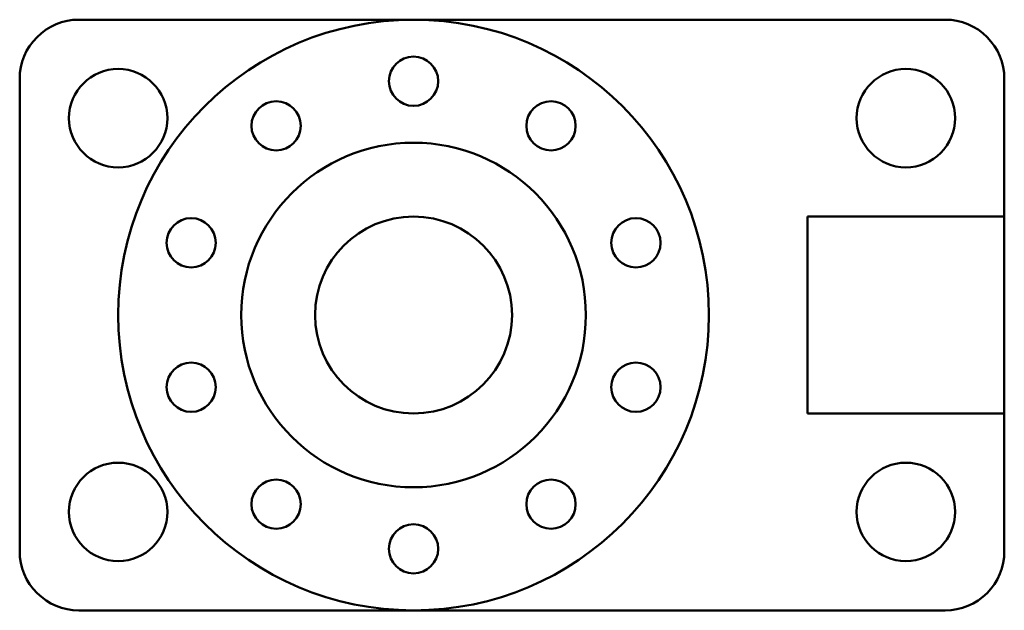
# Model space of a CAD drawing. Units: millimetres. Extents: x 2767 to 3480, y 0 to 1857.
# Tile 2 of 2: x 2767 to 2967, y 1737 to 1857. Entities that reach past the tile are written whole.
import ezdxf

# ---------------------------------------------------------------- set-up
doc = ezdxf.new("R2010")
doc.units = ezdxf.units.MM
doc.layers.add('M-OUTL', color=7, linetype='Continuous', lineweight=50)

# ---------------------------------------------------------------- blocks, each defined once
blk = doc.blocks.new('*U1')
blk.add_circle((0, 0), 5)
blk = doc.blocks.new('*U2')
at = {"layer": 'M-OUTL', "color": 0, "linetype": 'ByBlock', "lineweight": -2, "transparency": 16777216}
blk.add_blockref('*U1', (2847.32, 1844.34), dxfattribs=at)
for p, rotation in [((2819.4, 1835.27), 35.99999999999999), ((2875.24, 1835.27), 324), ((2802.14, 1811.52), 72), ((2892.49, 1811.52), 288), ((2802.14, 1782.17), 108), ((2892.49, 1782.17), 252), ((2819.4, 1758.42), 144), ((2875.24, 1758.42), 216), ((2847.32, 1749.34), 180)]:
    blk.add_blockref('*U1', p, dxfattribs=dict(at, rotation=rotation))

msp = doc.modelspace()

# ---------------------------------------------------------------- linework, layer by layer
at = {"layer": 'M-OUTL'}
for p, q in [((2967.32, 1816.84), (2927.32, 1816.84)), ((2927.32, 1816.84), (2927.32, 1776.84)), ((2967.32, 1816.84), (2967.32, 1776.84)), ((2967.32, 1776.84), (2927.32, 1776.84))]:
    msp.add_line(p, q, dxfattribs=at)
msp.add_lwpolyline([(2779.32, 1736.84), (2955.32, 1736.84, 0.414214), (2967.32, 1748.84), (2967.32, 1844.84, 0.414214), (2955.32, 1856.84), (2779.32, 1856.84, 0.414214), (2767.32, 1844.84), (2767.32, 1748.84, 0.414214)], format="xyb", close=True, dxfattribs=at)
for centre, radius in [((2847.32, 1796.84), 60), ((2787.32, 1836.84), 10), ((2947.32, 1836.84), 10), ((2847.32, 1796.84), 35), ((2847.32, 1796.84), 20), ((2787.32, 1756.84), 10), ((2947.32, 1756.84), 10)]:
    msp.add_circle(centre, radius, dxfattribs=at)

# ---------------------------------------------------------------- block references
msp.add_blockref('*U2', (0, 0), dxfattribs=at)

doc.saveas('drawing.dxf')
